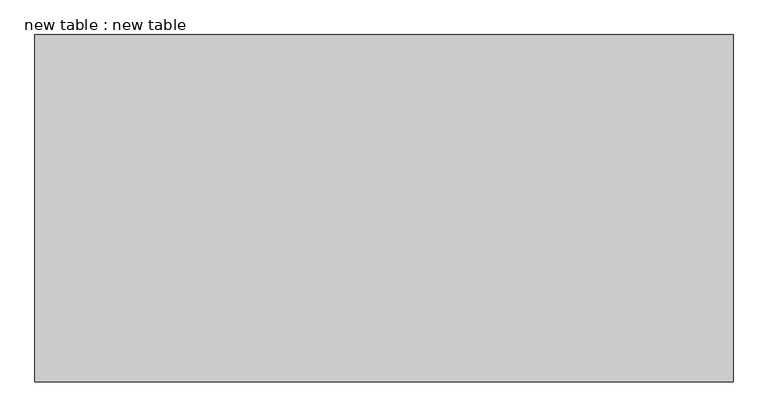
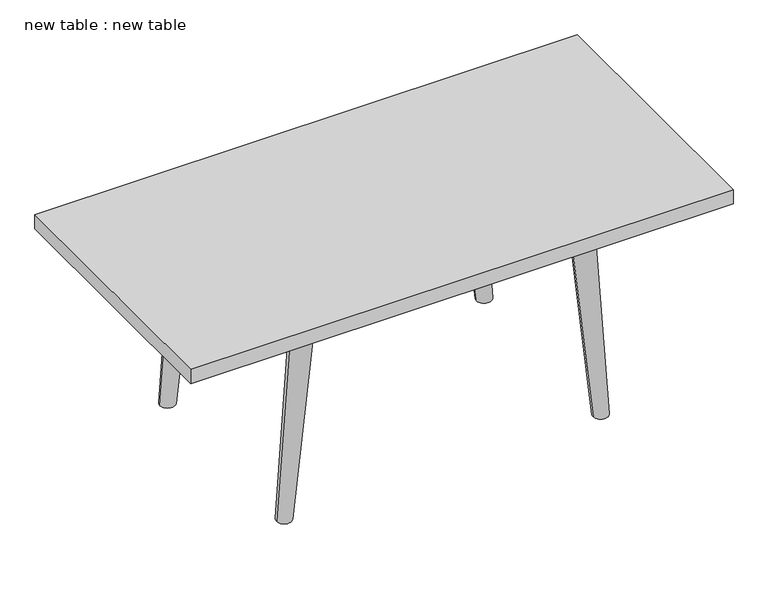
"""IFC4 building model written with IfcOpenShell, lengths in millimetres: furniture geometry, new table : new table."""

from ifc_helpers import new_model, si_unit, frame, origin, place, context, project, spatial, polyline, circle_curve, outline, extrude, source, transform, mapped, element, save
from ifc_brep_helpers import plane_surface, spline_surface, advanced_brep


def new_table_new_table_faa1bdb5(model_context):
    return source(origin(), model_context, "Body", "SolidModel", [
        extrude(outline(polyline([(915.0, 455.0), (915.0, -455.0), (-915.0, -455.0), (-915.0, 455.0), (915.0, 455.0)])), frame((0.0, 0.0, 685.8), z_axis=(0.0, 0.0, 1.0), x_axis=(1.0, 0.0, 0.0)), (0.0, 0.0, 1.0), 50.8),
        advanced_brep(
        [(-508.5274301, 340.7, 708.9845125), (-432.3274301, 340.7, 708.9845125), (-559.3274301, 340.7, 0.0), (-508.5274301, 340.7, 0.0)],
        [
            (0, 1, circle_curve(frame((-470.4274301, 340.7, 708.9845125), z_axis=(0.0, 0.0, 1.0), x_axis=(1.0, 0.0, 0.0)), 38.1)),
            (1, 0, circle_curve(frame((-470.4274301, 340.7, 708.9845125), z_axis=(0.0, 0.0, 1.0), x_axis=(1.0, 0.0, 0.0)), 38.1)),
            (2, 3, circle_curve(frame((-533.9274301, 340.7, 0.0), z_axis=(0.0, 0.0, -1.0), x_axis=(1.0, 0.0, 0.0)), 25.4)),
            (3, 2, circle_curve(frame((-533.9274301, 340.7, 0.0), z_axis=(0.0, 0.0, -1.0), x_axis=(1.0, 0.0, 0.0)), 25.4)),
            (3, 1),
            (0, 2),
        ],
        [
            plane_surface(frame((-470.4274301, 340.7, 708.9845125), z_axis=(0.0, 0.0, 1.0), x_axis=(0.0, -1.0, 0.0))),
            plane_surface(frame((-533.9274301, 340.7, 0.0), z_axis=(0.0, 0.0, -1.0), x_axis=(0.0, -1.0, 0.0))),
            spline_surface(2, 1, [[(-559.3274301, 340.7, 0.0), (-508.5274301, 340.7, 708.9845125)], [(-559.3274301, 315.3, 0.0), (-508.5274301, 302.59999999999997, 708.9845125)], [(-533.9274301, 315.3, 0.0), (-470.4274301, 302.59999999999997, 708.9845125)], [(-508.52743010000006, 315.29999999999995, 0.0), (-432.32743009999996, 302.5999999999999, 708.9845125)], [(-508.5274301, 340.7, 0.0), (-432.3274301, 340.7, 708.9845125)]], [3, 2, 3], [2, 2], [0.0, 1.0, 2.0], [0.0, 1.0], weights=[[1.0, 1.0], [0.7071067811865476, 0.7071067811865476], [1.0, 1.0], [0.707106781186547, 0.707106781186547], [1.0, 1.0]]),
            spline_surface(2, 1, [[(-508.5274301, 340.7, 0.0), (-432.3274301, 340.7, 708.9845125)], [(-508.5274301, 366.1, 0.0), (-432.3274301, 378.79999999999995, 708.9845125)], [(-533.9274301, 366.1, 0.0), (-470.4274301, 378.79999999999995, 708.9845125)], [(-559.3274301000001, 366.09999999999997, 0.0), (-508.52743009999995, 378.7999999999999, 708.9845125)], [(-559.3274301, 340.7, 0.0), (-508.5274301, 340.7, 708.9845125)]], [3, 2, 3], [2, 2], [0.0, 1.0, 2.0], [0.0, 1.0], weights=[[1.0, 1.0], [0.7071067811865476, 0.7071067811865476], [1.0, 1.0], [0.7071067811865481, 0.7071067811865481], [1.0, 1.0]]),
        ],
        [
            (0, [[1, 2]]),
            (1, [[3, 4]]),
            (2, [[-4, 5, -1, 6]]),
            (3, [[-3, -6, -2, -5]]),
        ],
    ),
        advanced_brep(
        [(508.5274301, 340.7, 708.9845125), (432.3274301, 340.7, 708.9845125), (559.3274301, 340.7, 0.0), (508.5274301, 340.7, 0.0)],
        [
            (0, 1, circle_curve(frame((470.4274301, 340.7, 708.9845125), z_axis=(0.0, 0.0, 1.0), x_axis=(-1.0, 0.0, 0.0)), 38.1)),
            (1, 0, circle_curve(frame((470.4274301, 340.7, 708.9845125), z_axis=(0.0, 0.0, 1.0), x_axis=(-1.0, 0.0, 0.0)), 38.1)),
            (2, 3, circle_curve(frame((533.9274301, 340.7, 0.0), z_axis=(0.0, 0.0, -1.0), x_axis=(-1.0, 0.0, 0.0)), 25.4)),
            (3, 2, circle_curve(frame((533.9274301, 340.7, 0.0), z_axis=(0.0, 0.0, -1.0), x_axis=(-1.0, 0.0, 0.0)), 25.4)),
            (2, 0),
            (1, 3),
        ],
        [
            plane_surface(frame((470.4274301, 340.7, 708.9845125), z_axis=(0.0, 0.0, 1.0), x_axis=(0.0, 1.0, 0.0))),
            plane_surface(frame((533.9274301, 340.7, 0.0), z_axis=(0.0, 0.0, -1.0), x_axis=(0.0, 1.0, 0.0))),
            spline_surface(2, 1, [[(508.5274301, 340.7, 0.0), (432.3274301, 340.7, 708.9845125)], [(508.5274301, 315.29999999999995, 0.0), (432.3274301, 302.6, 708.9845125)], [(533.9274301, 315.29999999999995, 0.0), (470.4274301, 302.6, 708.9845125)], [(559.3274301000001, 315.3, 0.0), (508.52743009999995, 302.6000000000001, 708.9845125)], [(559.3274301, 340.7, 0.0), (508.5274301, 340.7, 708.9845125)]], [3, 2, 3], [2, 2], [0.0, 1.0, 2.0], [0.0, 1.0], weights=[[1.0, 1.0], [0.7071067811865476, 0.7071067811865476], [1.0, 1.0], [0.7071067811865481, 0.7071067811865481], [1.0, 1.0]]),
            spline_surface(2, 1, [[(559.3274301, 340.7, 0.0), (508.5274301, 340.7, 708.9845125)], [(559.3274301, 366.09999999999997, 0.0), (508.5274301, 378.8, 708.9845125)], [(533.9274301, 366.09999999999997, 0.0), (470.4274301, 378.8, 708.9845125)], [(508.52743010000006, 366.1, 0.0), (432.32743009999996, 378.80000000000007, 708.9845125)], [(508.5274301, 340.7, 0.0), (432.3274301, 340.7, 708.9845125)]], [3, 2, 3], [2, 2], [0.0, 1.0, 2.0], [0.0, 1.0], weights=[[1.0, 1.0], [0.7071067811865476, 0.7071067811865476], [1.0, 1.0], [0.707106781186547, 0.707106781186547], [1.0, 1.0]]),
        ],
        [
            (0, [[1, 2]]),
            (1, [[3, 4]]),
            (2, [[-3, 5, -2, 6]]),
            (3, [[-4, -6, -1, -5]]),
        ],
    ),
        advanced_brep(
        [(-508.5274301, -340.7, 708.9845125), (-432.3274301, -340.7, 708.9845125), (-559.3274301, -340.7, 0.0), (-508.5274301, -340.7, 0.0)],
        [
            (0, 1, circle_curve(frame((-470.4274301, -340.7, 708.9845125), z_axis=(0.0, 0.0, 1.0), x_axis=(1.0, 0.0, 0.0)), 38.1)),
            (1, 0, circle_curve(frame((-470.4274301, -340.7, 708.9845125), z_axis=(0.0, 0.0, 1.0), x_axis=(1.0, 0.0, 0.0)), 38.1)),
            (2, 3, circle_curve(frame((-533.9274301, -340.7, 0.0), z_axis=(0.0, 0.0, -1.0), x_axis=(1.0, 0.0, 0.0)), 25.4)),
            (3, 2, circle_curve(frame((-533.9274301, -340.7, 0.0), z_axis=(0.0, 0.0, -1.0), x_axis=(1.0, 0.0, 0.0)), 25.4)),
            (2, 0),
            (1, 3),
        ],
        [
            plane_surface(frame((-470.4274301, -340.7, 708.9845125), z_axis=(0.0, 0.0, 1.0), x_axis=(0.0, -1.0, 0.0))),
            plane_surface(frame((-533.9274301, -340.7, 0.0), z_axis=(0.0, 0.0, -1.0), x_axis=(0.0, -1.0, 0.0))),
            spline_surface(2, 1, [[(-508.5274301, -340.7, 0.0), (-432.3274301, -340.7, 708.9845125)], [(-508.5274301, -315.29999999999995, 0.0), (-432.3274301, -302.6, 708.9845125)], [(-533.9274301, -315.29999999999995, 0.0), (-470.4274301, -302.6, 708.9845125)], [(-559.3274301000001, -315.3, 0.0), (-508.52743009999995, -302.6000000000001, 708.9845125)], [(-559.3274301, -340.7, 0.0), (-508.5274301, -340.7, 708.9845125)]], [3, 2, 3], [2, 2], [0.0, 1.0, 2.0], [0.0, 1.0], weights=[[1.0, 1.0], [0.7071067811865476, 0.7071067811865476], [1.0, 1.0], [0.7071067811865481, 0.7071067811865481], [1.0, 1.0]]),
            spline_surface(2, 1, [[(-559.3274301, -340.7, 0.0), (-508.5274301, -340.7, 708.9845125)], [(-559.3274301, -366.09999999999997, 0.0), (-508.5274301, -378.8, 708.9845125)], [(-533.9274301, -366.09999999999997, 0.0), (-470.4274301, -378.8, 708.9845125)], [(-508.52743010000006, -366.1, 0.0), (-432.32743009999996, -378.80000000000007, 708.9845125)], [(-508.5274301, -340.7, 0.0), (-432.3274301, -340.7, 708.9845125)]], [3, 2, 3], [2, 2], [0.0, 1.0, 2.0], [0.0, 1.0], weights=[[1.0, 1.0], [0.7071067811865476, 0.7071067811865476], [1.0, 1.0], [0.707106781186547, 0.707106781186547], [1.0, 1.0]]),
        ],
        [
            (0, [[1, 2]]),
            (1, [[3, 4]]),
            (2, [[-3, 5, -2, 6]]),
            (3, [[-4, -6, -1, -5]]),
        ],
    ),
        advanced_brep(
        [(508.5274301, -340.7, 685.8), (432.3274301, -340.7, 685.8), (559.3274301, -340.7, 0.0), (508.5274301, -340.7, 0.0)],
        [
            (0, 1, circle_curve(frame((470.4274301, -340.7, 685.8), z_axis=(0.0, 0.0, 1.0), x_axis=(-1.0, 0.0, 0.0)), 38.1)),
            (1, 0, circle_curve(frame((470.4274301, -340.7, 685.8), z_axis=(0.0, 0.0, 1.0), x_axis=(-1.0, 0.0, 0.0)), 38.1)),
            (2, 3, circle_curve(frame((533.9274301, -340.7, 0.0), z_axis=(0.0, 0.0, -1.0), x_axis=(-1.0, 0.0, 0.0)), 25.4)),
            (3, 2, circle_curve(frame((533.9274301, -340.7, 0.0), z_axis=(0.0, 0.0, -1.0), x_axis=(-1.0, 0.0, 0.0)), 25.4)),
            (3, 1),
            (0, 2),
        ],
        [
            plane_surface(frame((470.4274301, -340.7, 685.8), z_axis=(0.0, 0.0, 1.0), x_axis=(0.0, 1.0, 0.0))),
            plane_surface(frame((533.9274301, -340.7, 0.0), z_axis=(0.0, 0.0, -1.0), x_axis=(0.0, 1.0, 0.0))),
            spline_surface(2, 1, [[(559.3274301, -340.7, 0.0), (508.5274301, -340.7, 685.8)], [(559.3274301, -315.3, 0.0), (508.5274301, -302.59999999999997, 685.8)], [(533.9274301, -315.3, 0.0), (470.4274301, -302.59999999999997, 685.8)], [(508.52743010000006, -315.29999999999995, 0.0), (432.32743009999996, -302.5999999999999, 685.8)], [(508.5274301, -340.7, 0.0), (432.3274301, -340.7, 685.8)]], [3, 2, 3], [2, 2], [0.0, 1.0, 2.0], [0.0, 1.0], weights=[[1.0, 1.0], [0.7071067811865476, 0.7071067811865476], [1.0, 1.0], [0.707106781186547, 0.707106781186547], [1.0, 1.0]]),
            spline_surface(2, 1, [[(508.5274301, -340.7, 0.0), (432.3274301, -340.7, 685.8)], [(508.5274301, -366.1, 0.0), (432.3274301, -378.79999999999995, 685.8)], [(533.9274301, -366.1, 0.0), (470.4274301, -378.79999999999995, 685.8)], [(559.3274301000001, -366.09999999999997, 0.0), (508.52743009999995, -378.7999999999999, 685.8)], [(559.3274301, -340.7, 0.0), (508.5274301, -340.7, 685.8)]], [3, 2, 3], [2, 2], [0.0, 1.0, 2.0], [0.0, 1.0], weights=[[1.0, 1.0], [0.7071067811865476, 0.7071067811865476], [1.0, 1.0], [0.7071067811865481, 0.7071067811865481], [1.0, 1.0]]),
        ],
        [
            (0, [[1, 2]]),
            (1, [[3, 4]]),
            (2, [[-4, 5, -1, 6]]),
            (3, [[-3, -6, -2, -5]]),
        ],
    ),
    ])


if __name__ == "__main__":
    model = new_model("IFC4")
    model_context = context("Model", 3, world=origin())
    ifc_project = project(units=[si_unit("LENGTHUNIT", "METRE", prefix="MILLI")], contexts=[model_context])
    site = spatial("IfcSite", under=ifc_project)
    building = spatial("IfcBuilding", under=site)
    placement = place(None, origin())
    new_table_new_table_shape = new_table_new_table_faa1bdb5(model_context)
    element("IfcFurniture", 1, ObjectType="new table : new table", at=placement, inside=building, context=model_context, shape_type="MappedRepresentation", body=[
        mapped(new_table_new_table_shape, transform((0.0, 0.0, 0.0), x_axis=(1.0, 0.0, 0.0), y_axis=(0.0, 1.0, 0.0), z_axis=(0.0, 0.0, 1.0))),
    ])
    save(model, "model.ifc")

# Revit data of these elements
# Type "new table : new table"
#   Default Elevation = 0
# Element 1 (IfcFurniture, "new table : new table")
#   Materials on its faces: "table(1)", "table"
# Materials
#   "table(1)": class "Generic", colour RGB 120 120 120, transparency 0, Cost = 0
#   "table": class "Generic", colour RGB 120 120 120, transparency 0, Cost = 0
